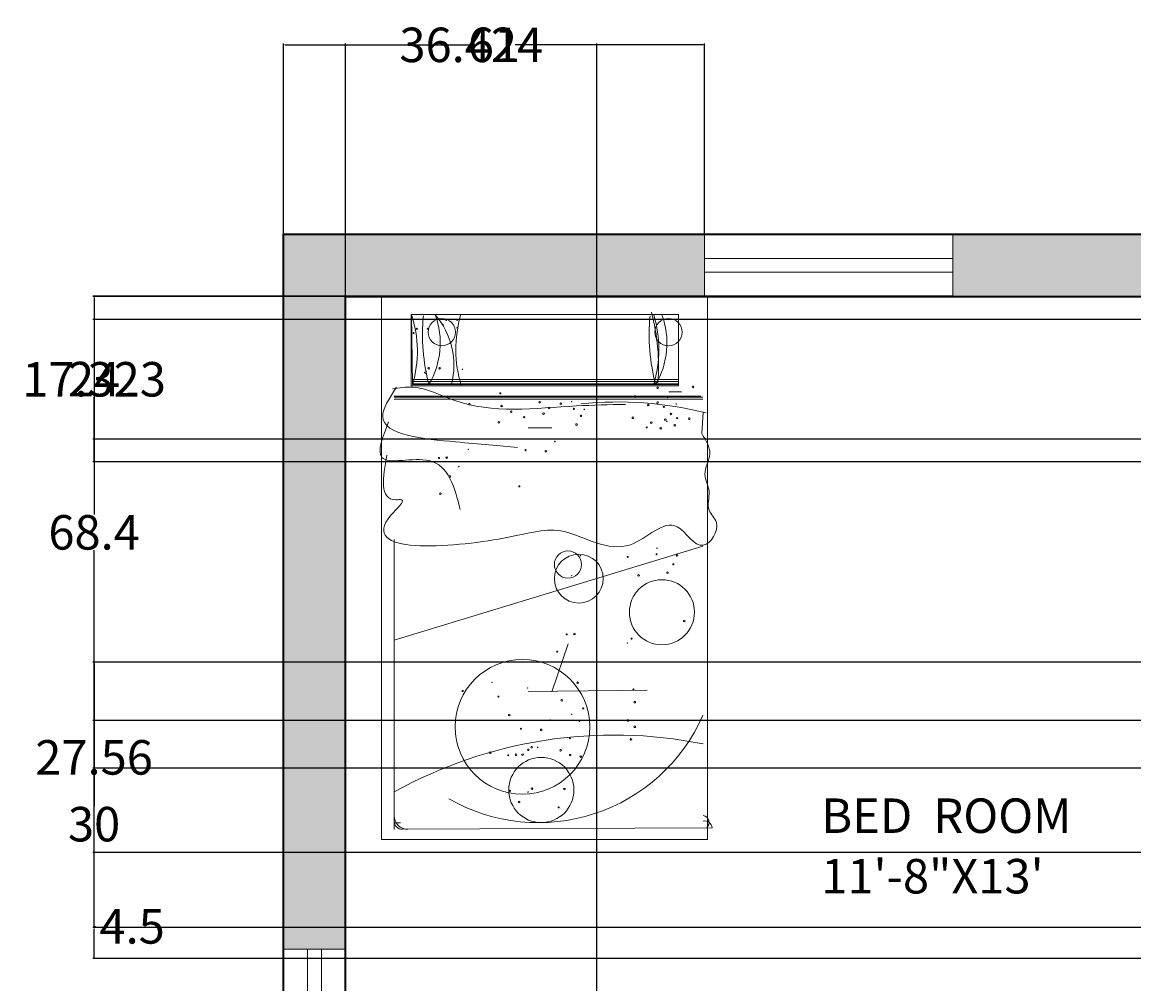
# Model space of a CAD drawing. Units: inches. Extents: x 2807 to 3326, y 2005 to 2580.
# Tile 9 of 12: x 2807 to 2968, y 2441 to 2580. Entities that reach past the tile are written whole.
import ezdxf

# ---------------------------------------------------------------- set-up
doc = ezdxf.new("R2010")
doc.units = ezdxf.units.IN
doc.header["$LTSCALE"] = 0.4
for name, color, linetype, lineweight in [('A-ANNO-DIMS', 2, 'Continuous', 18), ('A-AREA-IDEN', 5, 'Continuous', 18), ('A-WALL-PATT', 231, 'Continuous', 13), ('Furniture', 7, 'Continuous', 15), ('WALL', 233, 'Continuous', 35), ('WINDOWS', 132, 'Continuous', 18)]:
    doc.layers.add(name, color=color, linetype=linetype, lineweight=lineweight)
doc.styles.get("Standard").update_dxf_attribs({"font": 'txt', "height": 5})
doc.dimstyles.get("Standard").update_dxf_attribs({"dimtxt": 0.18, "dimasz": 0.18, "dimexe": 0.18, "dimexo": 0.0625, "dimgap": 0.09, "dimtad": 0, "dimtih": 1, "dimtoh": 1, "dimdec": 4, "dimzin": 0, "dimdsep": 46, "dimtxsty": 'Standard', "dimcen": 0.09, "dimadec": 0, "dimazin": 0, "dimtfac": 1, "dimtdec": 4, "dimtofl": 0, "dimtmove": 0, "dimatfit": 3, "dimfxl": 1, "dimtolj": 1, "dimtzin": 0, "dimarcsym": 0})

# ---------------------------------------------------------------- blocks, each defined once
blk = doc.blocks.new('WIN-36')
at = {"ltscale": 0.4}
for p, q in [((0, 36), (0, 0)), ((9, 36), (0, 36)), ((3.5, 36), (3.5, 0)), ((5.5, 36), (5.5, 0)), ((9, 0), (9, 36)), ((0, 0), (9, 0))]:
    blk.add_line(p, q, dxfattribs=at)
blk = doc.blocks.new('BED-SINGLE')
for p, q in [((-24.2, -78.74), (-24.2, 0)), ((23.05, 0), (-24.2, 0)), ((23.05, 0), (23.05, -78.74)), ((-19.91, -2.64), (18.85, -2.64)), ((-19.91, -12.97), (-19.91, -2.64)), ((-19.86, -2.65), (-19.71, -12.79)), ((18.85, -2.64), (18.85, -12.97)), ((-19.71, -12.07), (18.88, -12.07)), ((-19.71, -12.36), (18.88, -12.36)), ((-19.71, -12.66), (18.88, -12.66)), ((-19.71, -12.79), (18.88, -12.79)), ((-22.34, -14.47), (22.1, -14.45)), ((18.85, -12.97), (-19.91, -12.97)), ((19.29, -13.84), (17.45, -13.84)), ((-22.36, -14.62), (22.4, -14.6)), ((-22.36, -14.92), (22.4, -14.9)), ((22.21, -19.89), (22.42, -16.84)), ((0.5, -19.06), (-2.92, -19.06)), ((-22.34, -35.25), (-22.34, -77.26)), ((-22.34, -35.25), (-22.34, -75.28)), ((-22.36, -49.81), (22.4, -36.21)), ((-22.34, -50.11), (-22.34, -35.53)), ((2.87, -50.36), (0.49, -57.3)), ((14.32, -57.07), (-2.92, -57.29)), ((-22.21, -76.32), (-21.42, -76.32)), ((-21.16, -77.25), (23.72, -77.02)), ((23.05, -78.74), (-24.2, -78.74))]:
    blk.add_line(p, q)
for centre, radius in [((-15.45, -5.18), 1.97), ((-19.07, -4.7), 0.0787), ((-17.49, -4.7), 0.0787), ((-15.29, -4.08), 0.0394), ((-14.82, -3.45), 0.0394), ((-13.24, -3.45), 0.0394), ((-13.24, -4.55), 0.0394), ((17.4, -5.19), 1.97), ((-19.54, -5.33), 0.0787), ((-17.82, -11.05), 0.118), ((-17.35, -10.43), 0.118), ((-15.77, -10.43), 0.118), ((-12.46, -10.58), 0.0394), ((-6.97, -14.05), 0.0787), ((12.55, -14.52), 0.118), ((15.84, -13.26), 0.118), ((20.96, -13.12), 0.118), ((-11.46, -15.62), 0.118), ((-6.78, -15.9), 0.118), ((-1.26, -15.34), 0.118), ((0.11, -16.17), 0.118), ((1.8, -15.56), 0.118), ((14.47, -15.76), 0.118), ((15.82, -15.39), 0.118), ((16.73, -16.02), 0.0787), ((17.27, -14.65), 0.0394), ((18.52, -15.61), 0.0394), ((-5.4, -16.72), 0.118), ((-3.52, -17.51), 0.0787), ((-0.71, -17), 0.118), ((3.7, -16.3), 0.0787), ((4.72, -17.32), 0.118), ((5.19, -16.39), 0.0394), ((12.24, -17.6), 0.118), ((17.76, -17.04), 0.118), ((18.66, -17.64), 0.0787), ((20.41, -17.75), 0.118), ((-7.18, -18.26), 0.118), ((4.08, -18.58), 0.118), ((14.25, -19), 0.0787), ((14.9, -18.3), 0.118), ((16.28, -19.13), 0.118), ((16.93, -17.87), 0.118), ((17.15, -18.11), 0.0394), ((18.3, -18.69), 0.118), ((-11.61, -22.18), 0.0394), ((-3.31, -22.29), 0.0787), ((-0.37, -22.46), 0.118), ((0.94, -21.04), 0.0394), ((-15.86, -23.43), 0.0787), ((-14.74, -23.37), 0.118), ((-12.98, -24.68), 0.0394), ((-14.28, -26.11), 0.118), ((-15.65, -28.61), 0.118), ((-4.22, -27.54), 0.0787), ((2.83, -38.87), 1.97), ((15.74, -36.51), 0.0394), ((4.4, -40.91), 3.54), ((4.64, -37.58), 0.0394), ((11.49, -37.77), 0.0787), ((15.68, -37.38), 0.0787), ((18.63, -37.54), 0.118), ((17.26, -40.05), 0.118), ((18.11, -38.84), 0.0787), ((16.45, -45.79), 4.72), ((13.06, -40.44), 0.118), ((19.68, -47.06), 0.118), ((2.65, -49), 0.0787), ((3.77, -48.94), 0.118), ((12.05, -49.61), 0.0787), ((1.28, -51.5), 0.0787), ((11.44, -50.24), 0.0394), ((-3.76, -62.4), 9.76), ((-8.18, -55.94), 0.0394), ((4.23, -56), 0.118), ((-12.43, -57.2), 0.0787), ((-7.25, -58.02), 0.0787), ((-3, -56.76), 0.0394), ((12.32, -56.97), 0.0787), ((1.92, -58.54), 0.118), ((12.52, -58.82), 0.118), ((-5.68, -60.69), 0.118), ((5.04, -59.72), 0.0787), ((-3.99, -62.67), 0.0787), ((-1.05, -62.84), 0.118), ((0.26, -61.41), 0.0394), ((4.48, -61.53), 0.0787), ((11.5, -61.47), 0.118), ((12.52, -62.39), 0.118), ((3.11, -64.04), 0.0787), ((11.96, -64.21), 0.118), ((-8.43, -66.14), 0.118), ((-2.92, -65.73), 0.118), ((-2.42, -65.34), 0.118), ((-1.57, -65.38), 0.0394), ((1.77, -65.78), 0.118), ((-5.82, -66.51), 0.0787), ((-1.03, -71.55), 4.72), ((-4.7, -66.45), 0.118), ((-3.75, -66.42), 0.118), ((3.15, -66.47), 0.118), ((4.68, -66.71), 0.118), ((-5.61, -71.69), 0.118), ((-2.94, -71.86), 0.0394), ((-2.37, -71.35), 0.118), ((2.32, -71.4), 0.118), ((-4.24, -73.29), 0.118), ((1.48, -74.08), 0.0787)]:
    blk.add_circle(centre, radius)
for centre, radius, start, end in [((-35.51, -7.95), 16.53, 343.0006, 18.6759), ((10.58, -5.48), 28.83, 174.7074, 194.6885), ((-27.69, -6.75), 12.01, 329.8072, 19.9256), ((-25.06, -10.01), 11.36, 345.8396, 40.337), ((4.43, -7.67), 17.85, 163.6634, 197.1743), ((43.43, -5.5), 28.83, 174.7074, 194.6885), ((-14.89, -10.2), 30.85, 355.6161, 14.8863), ((-1.49, -7.71), 17.5, 343.1329, 16.7593), ((5.16, -6.76), 12.01, 329.8072, 19.9256), ((10.02, -67.77), 52.46, 75.8437, 95.7821), ((-1.46, -50.2), 26.08, 240.1506, 336.1931), ((9.49, -129.11), 65.53, 78.633, 119.0775), ((-20.37, -75.28), 1.97, 180, 270), ((22.26, -76.26), 1.02, 311.9337, 80.5378), ((-21.16, -76.07), 1.18, 180, 270), ((22.61, -77.16), 1.13, 7.0311, 99.2977)]:
    blk.add_arc(centre, radius, start, end)
for points, knots in [([(-22, -13.16), (-23.02, -14.71), (-26.47, -19.94), (-13.14, -21.11), (-7.15, -21.67), (-4.47, -21.92)], [0, 0, 0, 0, 4.712342, 15.867179, 24.91455, 24.91455, 24.91455, 24.91455]), ([(11.17, -15.66), (8.81, -15.7), (0.54, -15.87), (-10.21, -17.37), (-18.53, -12.79), (-21.61, -13.25), (-22.61, -13.4)], [0, 0, 0, 0, 7.121262, 24.909491, 31.123221, 34.101394, 34.101394, 34.101394, 34.101394]), ([(-23.16, -18.18), (-24, -20.34), (-25.96, -25.33), (-15.15, -21.84), (-13.61, -27.69), (-12.77, -30.9)], [0, 0, 0, 0, 5.247261, 12.129135, 20.530793, 20.530793, 20.530793, 20.530793]), ([(-23.42, -23.01), (-23.98, -26.23), (-24.61, -29.87), (-20.32, -29.28), (-30.03, -37.77), (-6.68, -35.83), (2.09, -32.61), (11.16, -38.92), (18.11, -30.55), (22.1, -38.17), (25.33, -33.01), (22.67, -30.96), (23.73, -28.27), (22.1, -25.67), (24.04, -22.75), (22.83, -20.86), (22.21, -19.89)], [0, 0, 0, 0, 6.608381, 7.436978, 10.160479, 26.82811, 35.651646, 45.441607, 52.697614, 57.347481, 61.162366, 63.231685, 65.951856, 68.505046, 71.545852, 74.730692, 74.730692, 74.730692, 74.730692])]:
    blk.add_open_spline(points, degree=3, knots=knots)
for p in [(3.38, -15.28), (3.38, -40.49), (3.38, -60.57)]:
    blk.add_point(p)
blk = doc.blocks.new('*D36')
at = {"layer": 'A-ANNO-DIMS', "color": 0, "lineweight": -2, "ltscale": 0.4, "transparency": 16777216}
for p, q in [((2844.57, 2549.64), (2844.57, 2577.21)), ((2844.75, 2577.03), (2872, 2577.03)), ((2905.39, 2577.03), (2878.13, 2577.03)), ((2905.57, 2549.64), (2905.57, 2577.21))]:
    blk.add_line(p, q, dxfattribs=at)
at = {"layer": 'A-ANNO-DIMS', "color": 0, "ltscale": 0.4, "transparency": 16777216}
for points in [[(2844.75, 2577.06), (2844.75, 2577), (2844.57, 2577.03)], [(2905.39, 2577.06), (2905.39, 2577), (2905.57, 2577.03)]]:
    blk.add_solid(points, dxfattribs=at)
at = {"layer": 'Defpoints', "color": 0, "ltscale": 0.4, "transparency": 16777216}
for p in [(2905.57, 2577.03), (2844.57, 2549.58), (2905.57, 2549.58)]:
    blk.add_point(p, dxfattribs=at)
at = {"layer": 'A-ANNO-DIMS', "color": 0, "ltscale": 0.4, "transparency": 16777216, "insert": (2875.07, 2577.03), "char_height": 5, "attachment_point": 5}
blk.add_mtext('\\A1;61', dxfattribs=at)
blk = doc.blocks.new('*D37')
at = {"layer": 'A-ANNO-DIMS', "color": 0, "lineweight": -2, "ltscale": 0.4, "transparency": 16777216}
for p, q in [((2853.567191, 2144.638996), (2853.567191, 2577.206496)), ((2853.747191, 2577.026496), (2859.189306, 2577.026496)), ((2889.811421, 2577.026496), (2884.369306, 2577.026496)), ((2889.991421, 2144.638996), (2889.991421, 2577.206496))]:
    blk.add_line(p, q, dxfattribs=at)
at = {"layer": 'A-ANNO-DIMS', "color": 0, "ltscale": 0.4, "transparency": 16777216}
for points in [[(2853.747191, 2577.056496), (2853.747191, 2576.996496), (2853.567191, 2577.026496)], [(2889.811421, 2577.056496), (2889.811421, 2576.996496), (2889.991421, 2577.026496)]]:
    blk.add_solid(points, dxfattribs=at)
at = {"layer": 'Defpoints', "color": 0, "ltscale": 0.4, "transparency": 16777216}
for p in [(2889.991421, 2577.026496), (2853.567191, 2144.576496), (2889.991421, 2144.576496)]:
    blk.add_point(p, dxfattribs=at)
at = {"layer": 'A-ANNO-DIMS', "color": 0, "ltscale": 0.4, "transparency": 16777216, "insert": (2871.779306, 2577.026496), "char_height": 5, "attachment_point": 5}
blk.add_mtext('\\A1;36.424', dxfattribs=at)
blk = doc.blocks.new('*D50')
at = {"layer": 'A-ANNO-DIMS', "color": 0, "lineweight": -2, "ltscale": 0.4, "transparency": 16777216}
for p, q in [((3139.504691, 2540.576496), (2816.937191, 2540.576496)), ((2817.117191, 2540.396496), (2817.117191, 2531.166496)), ((2817.117191, 2516.756496), (2817.117191, 2525.986496)), ((3139.504691, 2516.576496), (2816.937191, 2516.576496))]:
    blk.add_line(p, q, dxfattribs=at)
at = {"layer": 'A-ANNO-DIMS', "color": 0, "ltscale": 0.4, "transparency": 16777216}
for points in [[(2817.087191, 2540.396496), (2817.147191, 2540.396496), (2817.117191, 2540.576496)], [(2817.087191, 2516.756496), (2817.147191, 2516.756496), (2817.117191, 2516.576496)]]:
    blk.add_solid(points, dxfattribs=at)
at = {"layer": 'Defpoints', "color": 0, "ltscale": 0.4, "transparency": 16777216}
for p in [(2817.117191, 2540.576496), (3139.567191, 2540.576496), (3139.567191, 2516.576496)]:
    blk.add_point(p, dxfattribs=at)
at = {"layer": 'A-ANNO-DIMS', "color": 0, "ltscale": 0.4, "transparency": 16777216, "insert": (2817.117191, 2528.576496), "char_height": 5, "attachment_point": 5}
blk.add_mtext('\\A1;24', dxfattribs=at)
blk = doc.blocks.new('*D51')
at = {"layer": 'A-ANNO-DIMS', "color": 0, "lineweight": -2, "ltscale": 0.4, "transparency": 16777216}
for p, q in [((3135.004691, 2479.076496), (2816.937191, 2479.076496)), ((2817.117191, 2478.896496), (2817.117191, 2466.666496)), ((2817.117191, 2449.256496), (2817.117191, 2461.486496)), ((3135.004691, 2449.076496), (2816.937191, 2449.076496))]:
    blk.add_line(p, q, dxfattribs=at)
at = {"layer": 'A-ANNO-DIMS', "color": 0, "ltscale": 0.4, "transparency": 16777216}
for points in [[(2817.087191, 2478.896496), (2817.147191, 2478.896496), (2817.117191, 2479.076496)], [(2817.087191, 2449.256496), (2817.147191, 2449.256496), (2817.117191, 2449.076496)]]:
    blk.add_solid(points, dxfattribs=at)
at = {"layer": 'Defpoints', "color": 0, "ltscale": 0.4, "transparency": 16777216}
for p in [(2817.117191, 2479.076496), (3135.067191, 2479.076496), (3135.067191, 2449.076496)]:
    blk.add_point(p, dxfattribs=at)
at = {"layer": 'A-ANNO-DIMS', "color": 0, "ltscale": 0.4, "transparency": 16777216, "insert": (2817.117191, 2464.076496), "char_height": 5, "attachment_point": 5}
blk.add_mtext('\\A1;30', dxfattribs=at)
blk = doc.blocks.new('*D52')
at = {"layer": 'A-ANNO-DIMS', "color": 0, "lineweight": -2, "ltscale": 0.4, "transparency": 16777216}
for p, q in [((2941.5, 2540.58), (2816.94, 2540.58)), ((2817.12, 2540.4), (2817.12, 2508.96)), ((2817.12, 2472.35), (2817.12, 2503.78)), ((2995.79, 2472.17), (2816.94, 2472.17))]:
    blk.add_line(p, q, dxfattribs=at)
at = {"layer": 'A-ANNO-DIMS', "color": 0, "ltscale": 0.4, "transparency": 16777216}
for points in [[(2817.09, 2540.4), (2817.15, 2540.4), (2817.12, 2540.58)], [(2817.09, 2472.35), (2817.15, 2472.35), (2817.12, 2472.17)]]:
    blk.add_solid(points, dxfattribs=at)
at = {"layer": 'Defpoints', "color": 0, "ltscale": 0.4, "transparency": 16777216}
for p in [(2941.57, 2540.58), (2817.12, 2472.17), (2995.85, 2472.17)]:
    blk.add_point(p, dxfattribs=at)
at = {"layer": 'A-ANNO-DIMS', "color": 0, "ltscale": 0.4, "transparency": 16777216, "insert": (2817.12, 2506.37), "char_height": 5, "attachment_point": 5}
blk.add_mtext('\\A1;68.4', dxfattribs=at)
blk = doc.blocks.new('*D54')
at = {"layer": 'A-ANNO-DIMS', "color": 0, "lineweight": -2, "ltscale": 0.4, "transparency": 16777216}
for p, q in [((3198.393277, 2537.214927), (2816.937191, 2537.214927)), ((2817.117191, 2537.034927), (2817.117191, 2531.143527)), ((2817.117191, 2520.072127), (2817.117191, 2525.963527)), ((3198.393277, 2519.892127), (2816.937191, 2519.892127))]:
    blk.add_line(p, q, dxfattribs=at)
at = {"layer": 'A-ANNO-DIMS', "color": 0, "ltscale": 0.4, "transparency": 16777216}
for points in [[(2817.087191, 2537.034927), (2817.147191, 2537.034927), (2817.117191, 2537.214927)], [(2817.087191, 2520.072127), (2817.147191, 2520.072127), (2817.117191, 2519.892127)]]:
    blk.add_solid(points, dxfattribs=at)
at = {"layer": 'Defpoints', "color": 0, "ltscale": 0.4, "transparency": 16777216}
for p in [(2817.117191, 2537.214927), (3198.455777, 2537.214927), (3198.455777, 2519.892127)]:
    blk.add_point(p, dxfattribs=at)
at = {"layer": 'A-ANNO-DIMS', "color": 0, "ltscale": 0.4, "transparency": 16777216, "insert": (2817.117191, 2528.553527), "char_height": 5, "attachment_point": 5}
blk.add_mtext('\\A1;17.323', dxfattribs=at)
blk = doc.blocks.new('*D56')
at = {"layer": 'A-ANNO-DIMS', "color": 0, "lineweight": -2, "ltscale": 0.4, "transparency": 16777216}
for p, q in [((3258.250937, 2487.533633), (2816.937191, 2487.533633)), ((2817.117191, 2487.353633), (2817.117191, 2476.344133)), ((2817.117191, 2460.154633), (2817.117191, 2471.164133)), ((3258.250937, 2459.974633), (2816.937191, 2459.974633))]:
    blk.add_line(p, q, dxfattribs=at)
at = {"layer": 'A-ANNO-DIMS', "color": 0, "ltscale": 0.4, "transparency": 16777216}
for points in [[(2817.087191, 2487.353633), (2817.147191, 2487.353633), (2817.117191, 2487.533633)], [(2817.087191, 2460.154633), (2817.147191, 2460.154633), (2817.117191, 2459.974633)]]:
    blk.add_solid(points, dxfattribs=at)
at = {"layer": 'Defpoints', "color": 0, "ltscale": 0.4, "transparency": 16777216}
for p in [(2817.117191, 2487.533633), (3258.313437, 2487.533633), (3258.313437, 2459.974633)]:
    blk.add_point(p, dxfattribs=at)
at = {"layer": 'A-ANNO-DIMS', "color": 0, "ltscale": 0.4, "transparency": 16777216, "insert": (2817.117191, 2473.754133), "char_height": 5, "attachment_point": 5}
blk.add_mtext('\\A1;27.56', dxfattribs=at)
blk = doc.blocks.new('*D71')
at = {"layer": 'A-ANNO-DIMS', "color": 0, "lineweight": -2, "ltscale": 0.4, "transparency": 16777216}
for p, q in [((3139.5, 2449.08), (2816.94, 2449.08)), ((2817.12, 2449.08), (2817.12, 2449.26)), ((2817.12, 2449.26), (2817.3, 2449.26)), ((2817.12, 2444.76), (2817.12, 2448.9)), ((3139.5, 2444.58), (2816.94, 2444.58))]:
    blk.add_line(p, q, dxfattribs=at)
at = {"layer": 'A-ANNO-DIMS', "color": 0, "ltscale": 0.4, "transparency": 16777216}
for points in [[(2817.09, 2448.9), (2817.15, 2448.9), (2817.12, 2449.08)], [(2817.09, 2444.76), (2817.15, 2444.76), (2817.12, 2444.58)]]:
    blk.add_solid(points, dxfattribs=at)
at = {"layer": 'Defpoints', "color": 0, "ltscale": 0.4, "transparency": 16777216}
for p in [(2817.12, 2449.08), (3139.57, 2449.08), (3139.57, 2444.58)]:
    blk.add_point(p, dxfattribs=at)
at = {"layer": 'A-ANNO-DIMS', "color": 0, "ltscale": 0.4, "transparency": 16777216, "insert": (2822.63, 2449.26), "char_height": 5, "attachment_point": 5}
blk.add_mtext('\\A1;4.5', dxfattribs=at)

msp = doc.modelspace()

# ---------------------------------------------------------------- hatches: boundary and pattern name
at = {"layer": 'A-WALL-PATT', "ltscale": 0.4}
h = msp.add_hatch(color=256, dxfattribs=at)
h.dxf.hatch_style = 1
h.paths.add_polyline_path([(3288.5672, 2549.5765), (2941.5672, 2549.5765), (2941.5672, 2540.5765), (2993.5672, 2540.5765), (2993.5672, 2489.5693), (2998.0672, 2489.5693), (2998.0672, 2540.5765), (3135.0672, 2540.5765), (3135.0672, 2479.0765), (3139.5672, 2479.0765), (3139.5672, 2540.5765), (3279.5672, 2540.5765), (3279.5672, 2510.5765), (3288.5672, 2510.5765)])
h.paths.add_polyline_path([(2905.5672, 2549.5765), (2844.5672, 2549.5765), (2844.5672, 2445.94), (2853.5672, 2445.94), (2853.5672, 2540.5765), (2905.5672, 2540.5765)])
h.paths.add_polyline_path([(2853.5672, 2409.94), (2844.5672, 2409.94), (2844.5672, 2371.3497), (2853.5672, 2371.3497), (2853.5672, 2380.0765), (2909.0672, 2380.0765), (2909.0672, 2384.5765), (2853.5672, 2384.5765)])
h.paths.add_polyline_path([(2998.0672, 2389.0765), (2993.5672, 2389.0765), (2993.5672, 2384.5765), (2939.0672, 2384.5765), (2939.0672, 2380.0765), (2943.5672, 2380.0765), (2943.5672, 2314.0765), (2948.0672, 2314.0765), (2948.0672, 2380.0765), (2998.0672, 2380.0765)])
h.paths.add_polyline_path([(2998.0672, 2471.8029), (2993.5672, 2471.8029), (2993.5672, 2425.0765), (2998.0672, 2425.0765)])
h.paths.add_polyline_path([(2953.0672, 2279.5765), (2948.0672, 2279.5765), (2948.0672, 2284.0765), (2943.5672, 2284.0765), (2943.5672, 2279.5765), (2853.5672, 2279.5765), (2853.5672, 2289.0663), (2844.5672, 2289.0663), (2844.5672, 2227.8961), (2853.5672, 2227.8961), (2853.5672, 2275.0765), (2953.0672, 2275.0765)])
h.paths.add_polyline_path([(2943.5672, 2332.0765), (2853.5672, 2332.0765), (2853.5672, 2347.3497), (2844.5672, 2347.3497), (2844.5672, 2313.0663), (2853.5672, 2313.0663), (2853.5672, 2327.5765), (2943.5672, 2327.5765)])
h.paths.add_polyline_path([(3144.0672, 2279.5765), (2993.5672, 2279.5765), (2989.0672, 2279.5765), (2989.0672, 2275.0765), (2993.5672, 2275.0765), (2993.5672, 2144.5765), (2984.5672, 2144.5765), (2984.5672, 2135.5765), (2993.5672, 2135.5765), (2993.5672, 2120.0765), (3036.5672, 2120.0765), (3036.5672, 2129.0765), (2998.0672, 2129.0765), (2998.0672, 2275.0765), (3135.0672, 2275.0765), (3135.0672, 2129.0765), (3096.5672, 2129.0765), (3096.5672, 2120.0765), (3139.5672, 2120.0765), (3139.5672, 2135.5765), (3148.5672, 2135.5765), (3148.5672, 2144.5765), (3139.5672, 2144.5765), (3139.5672, 2275.0765), (3144.0672, 2275.0765)])
h.paths.add_polyline_path([(2984.5672, 2144.5765), (2925.9914, 2144.5765), (2925.9914, 2135.5765), (2984.5672, 2135.5765)])
h.paths.add_polyline_path([(2889.9914, 2144.5765), (2853.5672, 2144.5765), (2853.5672, 2191.8961), (2844.5672, 2191.8961), (2844.5672, 2135.5765), (2889.9914, 2135.5765)])
h.paths.add_polyline_path([(3196.0672, 2144.5765), (3148.5672, 2144.5765), (3148.5672, 2135.5765), (3196.0672, 2135.5765)])
h.paths.add_polyline_path([(3288.5672, 2191.8265), (3279.5672, 2191.8265), (3279.5672, 2144.5765), (3232.0672, 2144.5765), (3232.0672, 2135.5765), (3288.5672, 2135.5765)])
h.paths.add_polyline_path([(3288.5672, 2292.8229), (3279.5672, 2292.8229), (3279.5672, 2291.4371), (3279.5672, 2279.5765), (3189.5672, 2279.5765), (3189.5672, 2293.0765), (3185.0672, 2293.0765), (3185.0672, 2279.5765), (3180.0672, 2279.5765), (3180.0672, 2275.0765), (3279.5672, 2275.0765), (3279.5672, 2227.8265), (3288.5672, 2227.8265)])
h.paths.add_polyline_path([(3288.5672, 2368.0765), (3279.5672, 2368.0765), (3279.5672, 2332.0765), (3174.0672, 2332.0765), (3174.0672, 2327.5765), (3185.0672, 2327.5765), (3189.5672, 2327.5765), (3279.5672, 2327.5765), (3279.5672, 2316.8229), (3288.5672, 2316.8229)])
h.paths.add_polyline_path([(3288.5672, 2474.5765), (3279.5672, 2474.5765), (3279.5672, 2444.5765), (3139.5672, 2444.5765), (3139.5672, 2449.0765), (3135.0672, 2449.0765), (3135.0672, 2327.5765), (3144.0672, 2327.5765), (3144.0672, 2332.0765), (3139.5672, 2332.0765), (3139.5672, 2440.0765), (3279.5672, 2440.0765), (3279.5672, 2404.0765), (3288.5672, 2404.0765)])

# ---------------------------------------------------------------- linework, layer by layer
at = {"layer": 'WALL'}
for p, q in [((2844.5672, 2549.5765), (3288.5672, 2549.5765)), ((2844.5672, 2135.5765), (2844.5672, 2549.5765)), ((2853.5672, 2540.5765), (2993.5672, 2540.5765)), ((2853.5672, 2384.5765), (2853.5672, 2540.5765))]:
    msp.add_line(p, q, dxfattribs=at)

# ---------------------------------------------------------------- block references
at = {"layer": 'Furniture'}
msp.add_blockref('BED-SINGLE', (2882.9625, 2540.576), dxfattribs=at)
at = {"layer": 'WINDOWS', "rotation": 270}
msp.add_blockref('WIN-36', (2905.5672, 2549.5765), dxfattribs=at)
at = {"layer": 'WINDOWS'}
msp.add_blockref('WIN-36', (2844.5672, 2409.94), dxfattribs=at)

# ---------------------------------------------------------------- texts
at = {"layer": 'A-AREA-IDEN', "ltscale": 0.4}
for s, p in [('BED  ROOM', (2922.5058, 2462.8025)), ('11\'-8"X13\'', (2922.5058, 2454.0286))]:
    msp.add_text(s, height=5, dxfattribs=at).set_placement(p)

# ---------------------------------------------------------------- dimensions: what is measured, and where the dimension line sits
at = {"layer": 'A-ANNO-DIMS', "ltscale": 0.4}
for base, p1, p2, override, picture, middle in [((2905.5672, 2577.0265), (2844.5672, 2549.5765), (2905.5672, 2549.5765), {"dimdec": 0, "dimlfac": 1, "dimrnd": 0, "dimzin": 0, "dimdsep": 46, "dimlunit": 2}, '*D36', (2875.0672, 2577.0265)), ((2889.9914, 2577.0265), (2853.5672, 2144.5765), (2889.9914, 2144.5765), {"dimdec": 3, "dimlfac": 1, "dimrnd": 0, "dimzin": 0, "dimdsep": 46, "dimlunit": 2}, '*D37', (2871.7793, 2577.0265))]:
    dim = msp.add_linear_dim(base=base, p1=p1, p2=p2, dimstyle='Standard', override=override, dxfattribs=at)
    dim.commit()
    dim.dimension.update_dxf_attribs({"geometry": picture, "text_midpoint": middle})
for base, p1, p2, override, picture, middle in [((2817.1172, 2472.1697), (2941.5672, 2540.5765), (2995.85, 2472.1697), {"dimdec": 1, "dimlfac": 1, "dimrnd": 0, "dimzin": 0, "dimdsep": 46, "dimlunit": 2}, '*D52', (2817.1172, 2506.3731)), ((2817.1172, 2540.5765), (3139.5672, 2516.5765), (3139.5672, 2540.5765), {"dimdec": 0, "dimlfac": 1, "dimrnd": 0, "dimzin": 0, "dimdsep": 46, "dimlunit": 2}, '*D50', (2817.1172, 2528.5765)), ((2817.1172, 2537.2149), (3198.4558, 2519.8921), (3198.4558, 2537.2149), {"dimdec": 3, "dimlfac": 1, "dimrnd": 0, "dimzin": 0, "dimdsep": 46, "dimlunit": 2}, '*D54', (2817.1172, 2528.5535)), ((2817.1172, 2487.5336), (3258.3134, 2459.9746), (3258.3134, 2487.5336), {"dimdec": 2, "dimlfac": 1, "dimrnd": 0, "dimzin": 0, "dimdsep": 46, "dimlunit": 2}, '*D56', (2817.1172, 2473.7541)), ((2817.1172, 2479.0765), (3135.0672, 2449.0765), (3135.0672, 2479.0765), {"dimdec": 0, "dimlfac": 1, "dimrnd": 0, "dimzin": 0, "dimdsep": 46, "dimlunit": 2}, '*D51', (2817.1172, 2464.0765)), ((2817.1172, 2449.0765), (3139.5672, 2444.5765), (3139.5672, 2449.0765), {"dimdec": 1, "dimlfac": 1, "dimrnd": 0, "dimzin": 0, "dimdsep": 46, "dimlunit": 2}, '*D71', (2822.6253, 2449.2565))]:
    dim = msp.add_linear_dim(base=base, p1=p1, p2=p2, angle=90, dimstyle='Standard', override=override, dxfattribs=at)
    dim.commit()
    dim.dimension.update_dxf_attribs({"geometry": picture, "text_midpoint": middle})

doc.saveas('drawing.dxf')
